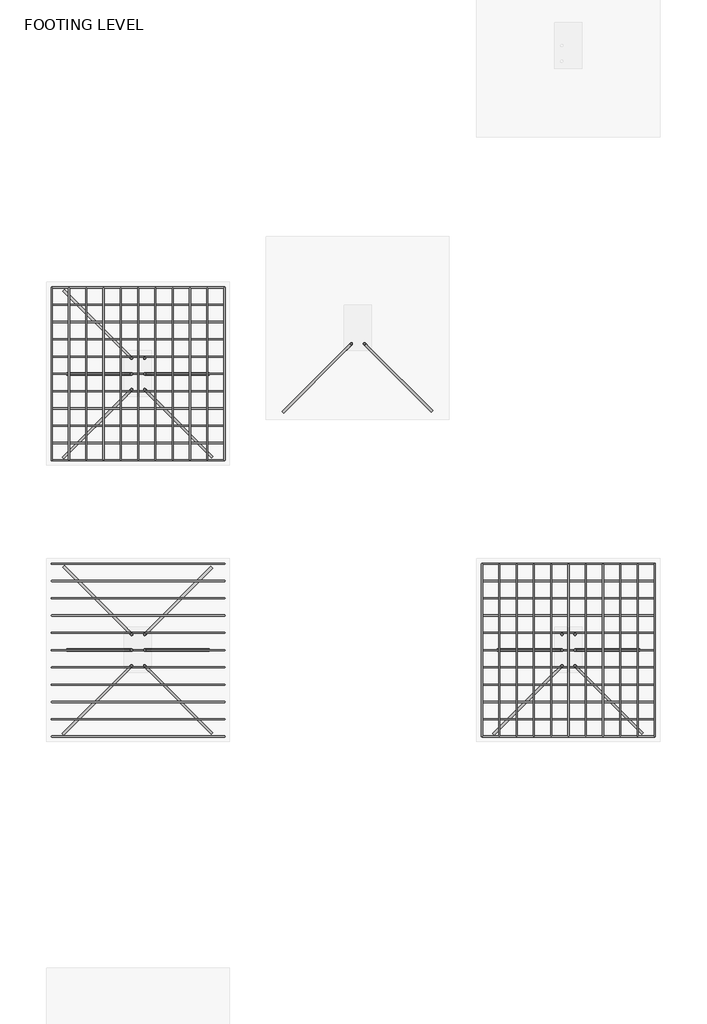
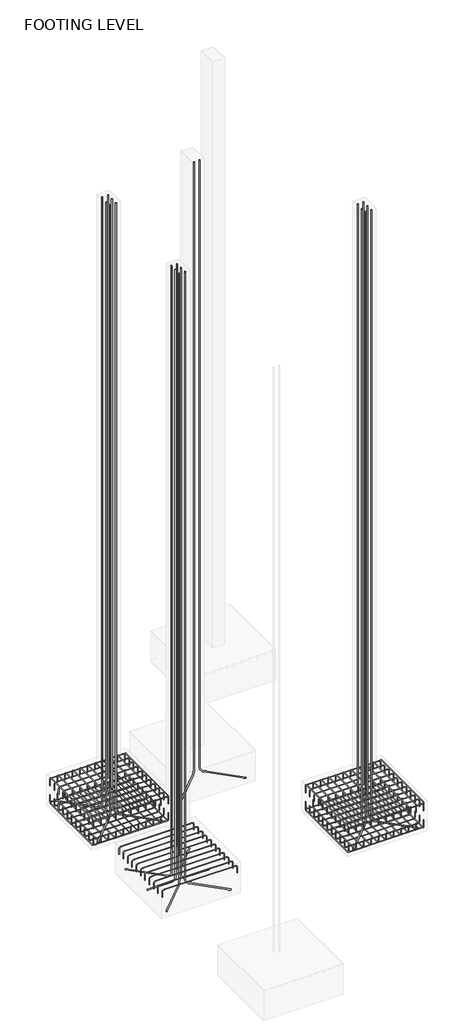
# One storey, part 6 of 10: 35 reinforcing bars.
"""IFC4 building model written with IfcOpenShell, lengths in millimetres."""

from ifc_helpers import new_model, si_unit, point, frame, origin, place, context, project, spatial, polyline, circle_curve, trimmed, segment, composite_curve, source, transform, mapped, element, save
from ifc_brep_helpers import swept_disk

model = new_model("IFC4")

# Units and contexts
model_context = context("Model", 3, world=origin())
ifc_project = project(units=[si_unit("LENGTHUNIT", "METRE", prefix="MILLI")], contexts=[model_context])

# Site, building, storey
site = spatial("IfcSite", under=ifc_project)
building = spatial("IfcBuilding", under=site)
storey = spatial("IfcBuildingStorey", under=building, Name="FOOTING LEVEL", Elevation=-1371.6)

# Reinforcing bars
placement = place(None, origin())
reinforcing_bar_shape = source(origin(), model_context, "Body", "SolidModel", [
    swept_disk(composite_curve([segment(polyline([(-3449.2793223, 2952.1203802, -1562.1), (-3449.2793223, 2952.1203802, -1447.8)]), True, "CONTINUOUS"), segment(trimmed(circle_curve(frame((-3449.2793223, 2985.4578802, -1447.8), z_axis=(-1.0, 0.0, 0.0), x_axis=(0.0, -33.33750000000009, 0.0)), 33.3375), [point((-3449.2793223, 2952.1203802, -1447.8))], [point((-3449.2793223, 2985.4578802, -1414.4625))], True, "CARTESIAN"), True, "CONTINUOUS"), segment(polyline([(-3449.2793223, 2985.4578802, -1414.4625), (-3449.2793223, 4357.0578802, -1414.4625)]), True, "CONTINUOUS"), segment(trimmed(circle_curve(frame((-3449.2793223, 4357.0578802, -1447.8), z_axis=(-1.0, 0.0, 0.0), x_axis=(0.0, 0.0, 33.337499999999864)), 33.3375), [point((-3449.2793223, 4357.0578802, -1414.4625))], [point((-3449.2793223, 4390.3953802, -1447.8))], True, "CARTESIAN"), True, "CONTINUOUS"), segment(polyline([(-3449.2793223, 4390.3953802, -1447.8), (-3449.2793223, 4390.3953802, -1562.1)]), True, "CONTINUOUS")], self_intersect=False), 4.7625),
])
element("IfcReinforcingBar", 1, at=placement, inside=storey, context=model_context, shape_type="MappedRepresentation", body=[
    mapped(reinforcing_bar_shape, transform((0.0, 0.0, 0.0), x_axis=(1.0, 0.0, 0.0), y_axis=(0.0, 1.0, 0.0), z_axis=(0.0, 0.0, 1.0))),
    mapped(reinforcing_bar_shape, transform((143.8275, 0.0, 0.0), x_axis=(1.0, 0.0, 0.0), y_axis=(0.0, 1.0, 0.0), z_axis=(0.0, 0.0, 1.0))),
    mapped(reinforcing_bar_shape, transform((287.655, 0.0, 0.0), x_axis=(1.0, 0.0, 0.0), y_axis=(0.0, 1.0, 0.0), z_axis=(0.0, 0.0, 1.0))),
    mapped(reinforcing_bar_shape, transform((431.4825, 0.0, 0.0), x_axis=(1.0, 0.0, 0.0), y_axis=(0.0, 1.0, 0.0), z_axis=(0.0, 0.0, 1.0))),
    mapped(reinforcing_bar_shape, transform((575.31, 0.0, 0.0), x_axis=(1.0, 0.0, 0.0), y_axis=(0.0, 1.0, 0.0), z_axis=(0.0, 0.0, 1.0))),
    mapped(reinforcing_bar_shape, transform((719.1375, 0.0, 0.0), x_axis=(1.0, 0.0, 0.0), y_axis=(0.0, 1.0, 0.0), z_axis=(0.0, 0.0, 1.0))),
    mapped(reinforcing_bar_shape, transform((862.965, 0.0, 0.0), x_axis=(1.0, 0.0, 0.0), y_axis=(0.0, 1.0, 0.0), z_axis=(0.0, 0.0, 1.0))),
    mapped(reinforcing_bar_shape, transform((1006.7925, 0.0, 0.0), x_axis=(1.0, 0.0, 0.0), y_axis=(0.0, 1.0, 0.0), z_axis=(0.0, 0.0, 1.0))),
    mapped(reinforcing_bar_shape, transform((1150.62, 0.0, 0.0), x_axis=(1.0, 0.0, 0.0), y_axis=(0.0, 1.0, 0.0), z_axis=(0.0, 0.0, 1.0))),
    mapped(reinforcing_bar_shape, transform((1294.4475, 0.0, 0.0), x_axis=(1.0, 0.0, 0.0), y_axis=(0.0, 1.0, 0.0), z_axis=(0.0, 0.0, 1.0))),
    mapped(reinforcing_bar_shape, transform((1438.275, 0.0, 0.0), x_axis=(1.0, 0.0, 0.0), y_axis=(0.0, 1.0, 0.0), z_axis=(0.0, 0.0, 1.0))),
])
reinforcing_bar_2_shape = source(origin(), model_context, "Body", "SolidModel", [
    swept_disk(composite_curve([segment(polyline([(-3449.2793223, 4390.3953802, -1790.7), (-3449.2793223, 4390.3953802, -1905.0)]), True, "CONTINUOUS"), segment(trimmed(circle_curve(frame((-3449.2793223, 4357.0578802, -1905.0), z_axis=(-1.0, 0.0, 0.0), x_axis=(0.0, 33.337499999999636, 0.0)), 33.3375), [point((-3449.2793223, 4390.3953802, -1905.0))], [point((-3449.2793223, 4357.0578802, -1938.3375))], True, "CARTESIAN"), True, "CONTINUOUS"), segment(polyline([(-3449.2793223, 4357.0578802, -1938.3375), (-3449.2793223, 2985.4578802, -1938.3375)]), True, "CONTINUOUS"), segment(trimmed(circle_curve(frame((-3449.2793223, 2985.4578802, -1905.0), z_axis=(-1.0, 0.0, 0.0), x_axis=(0.0, 0.0, -33.33750000000009)), 33.3375), [point((-3449.2793223, 2985.4578802, -1938.3375))], [point((-3449.2793223, 2952.1203802, -1905.0))], True, "CARTESIAN"), True, "CONTINUOUS"), segment(polyline([(-3449.2793223, 2952.1203802, -1905.0), (-3449.2793223, 2952.1203802, -1790.7)]), True, "CONTINUOUS")], self_intersect=False), 4.7625),
])
element("IfcReinforcingBar", 2, at=placement, inside=storey, context=model_context, shape_type="MappedRepresentation", body=[
    mapped(reinforcing_bar_2_shape, transform((0.0, 0.0, 0.0), x_axis=(1.0, 0.0, 0.0), y_axis=(0.0, 1.0, 0.0), z_axis=(0.0, 0.0, 1.0))),
    mapped(reinforcing_bar_2_shape, transform((143.8275, 0.0, 0.0), x_axis=(1.0, 0.0, 0.0), y_axis=(0.0, 1.0, 0.0), z_axis=(0.0, 0.0, 1.0))),
    mapped(reinforcing_bar_2_shape, transform((287.655, 0.0, 0.0), x_axis=(1.0, 0.0, 0.0), y_axis=(0.0, 1.0, 0.0), z_axis=(0.0, 0.0, 1.0))),
    mapped(reinforcing_bar_2_shape, transform((431.4825, 0.0, 0.0), x_axis=(1.0, 0.0, 0.0), y_axis=(0.0, 1.0, 0.0), z_axis=(0.0, 0.0, 1.0))),
    mapped(reinforcing_bar_2_shape, transform((575.31, 0.0, 0.0), x_axis=(1.0, 0.0, 0.0), y_axis=(0.0, 1.0, 0.0), z_axis=(0.0, 0.0, 1.0))),
    mapped(reinforcing_bar_2_shape, transform((719.1375, 0.0, 0.0), x_axis=(1.0, 0.0, 0.0), y_axis=(0.0, 1.0, 0.0), z_axis=(0.0, 0.0, 1.0))),
    mapped(reinforcing_bar_2_shape, transform((862.965, 0.0, 0.0), x_axis=(1.0, 0.0, 0.0), y_axis=(0.0, 1.0, 0.0), z_axis=(0.0, 0.0, 1.0))),
    mapped(reinforcing_bar_2_shape, transform((1006.7925, 0.0, 0.0), x_axis=(1.0, 0.0, 0.0), y_axis=(0.0, 1.0, 0.0), z_axis=(0.0, 0.0, 1.0))),
    mapped(reinforcing_bar_2_shape, transform((1150.62, 0.0, 0.0), x_axis=(1.0, 0.0, 0.0), y_axis=(0.0, 1.0, 0.0), z_axis=(0.0, 0.0, 1.0))),
    mapped(reinforcing_bar_2_shape, transform((1294.4475, 0.0, 0.0), x_axis=(1.0, 0.0, 0.0), y_axis=(0.0, 1.0, 0.0), z_axis=(0.0, 0.0, 1.0))),
    mapped(reinforcing_bar_2_shape, transform((1438.275, 0.0, 0.0), x_axis=(1.0, 0.0, 0.0), y_axis=(0.0, 1.0, 0.0), z_axis=(0.0, 0.0, 1.0))),
])
reinforcing_bar_3_shape = source(origin(), model_context, "Body", "SolidModel", [
    swept_disk(composite_curve([segment(polyline([(-2011.0043223, 4390.3953802, -1770.864029), (-2011.0043223, 4390.3953802, -1885.164029)]), True, "CONTINUOUS"), segment(trimmed(circle_curve(frame((-2044.3418223, 4390.3953802, -1885.164029), z_axis=(0.0, 1.0, 0.0), x_axis=(33.33750000000009, 0.0, 0.0)), 33.3375), [point((-2011.0043223, 4390.3953802, -1885.164029))], [point((-2044.3418223, 4390.3953802, -1918.501529))], True, "CARTESIAN"), True, "CONTINUOUS"), segment(polyline([(-2044.3418223, 4390.3953802, -1918.501529), (-3415.9418223, 4390.3953802, -1918.501529)]), True, "CONTINUOUS"), segment(trimmed(circle_curve(frame((-3415.9418223, 4390.3953802, -1885.164029), z_axis=(0.0, 1.0, 0.0), x_axis=(0.0, 0.0, -33.337499999999864)), 33.3375), [point((-3415.9418223, 4390.3953802, -1918.501529))], [point((-3449.2793223, 4390.3953802, -1885.164029))], True, "CARTESIAN"), True, "CONTINUOUS"), segment(polyline([(-3449.2793223, 4390.3953802, -1885.164029), (-3449.2793223, 4390.3953802, -1770.864029)]), True, "CONTINUOUS")], self_intersect=False), 4.7625),
])
element("IfcReinforcingBar", 3, at=placement, inside=storey, context=model_context, shape_type="MappedRepresentation", body=[
    mapped(reinforcing_bar_3_shape, transform((0.0, 0.0, 0.0), x_axis=(1.0, 0.0, 0.0), y_axis=(0.0, 1.0, 0.0), z_axis=(0.0, 0.0, 1.0))),
    mapped(reinforcing_bar_3_shape, transform((0.0, -143.8275, 0.0), x_axis=(1.0, 0.0, 0.0), y_axis=(0.0, 1.0, 0.0), z_axis=(0.0, 0.0, 1.0))),
    mapped(reinforcing_bar_3_shape, transform((0.0, -287.655, 0.0), x_axis=(1.0, 0.0, 0.0), y_axis=(0.0, 1.0, 0.0), z_axis=(0.0, 0.0, 1.0))),
    mapped(reinforcing_bar_3_shape, transform((0.0, -431.4825, 0.0), x_axis=(1.0, 0.0, 0.0), y_axis=(0.0, 1.0, 0.0), z_axis=(0.0, 0.0, 1.0))),
    mapped(reinforcing_bar_3_shape, transform((0.0, -575.31, 0.0), x_axis=(1.0, 0.0, 0.0), y_axis=(0.0, 1.0, 0.0), z_axis=(0.0, 0.0, 1.0))),
    mapped(reinforcing_bar_3_shape, transform((0.0, -719.1375, 0.0), x_axis=(1.0, 0.0, 0.0), y_axis=(0.0, 1.0, 0.0), z_axis=(0.0, 0.0, 1.0))),
    mapped(reinforcing_bar_3_shape, transform((0.0, -862.965, 0.0), x_axis=(1.0, 0.0, 0.0), y_axis=(0.0, 1.0, 0.0), z_axis=(0.0, 0.0, 1.0))),
    mapped(reinforcing_bar_3_shape, transform((0.0, -1006.7925, 0.0), x_axis=(1.0, 0.0, 0.0), y_axis=(0.0, 1.0, 0.0), z_axis=(0.0, 0.0, 1.0))),
    mapped(reinforcing_bar_3_shape, transform((0.0, -1150.62, 0.0), x_axis=(1.0, 0.0, 0.0), y_axis=(0.0, 1.0, 0.0), z_axis=(0.0, 0.0, 1.0))),
    mapped(reinforcing_bar_3_shape, transform((0.0, -1294.4475, 0.0), x_axis=(1.0, 0.0, 0.0), y_axis=(0.0, 1.0, 0.0), z_axis=(0.0, 0.0, 1.0))),
    mapped(reinforcing_bar_3_shape, transform((0.0, -1438.275, 0.0), x_axis=(1.0, 0.0, 0.0), y_axis=(0.0, 1.0, 0.0), z_axis=(0.0, 0.0, 1.0))),
])
reinforcing_bar_4_shape = source(origin(), model_context, "Body", "SolidModel", [
    swept_disk(composite_curve([segment(polyline([(-2011.0043223, 2952.1203802, -1586.5406765), (-2011.0043223, 2952.1203802, -1472.2406765)]), True, "CONTINUOUS"), segment(trimmed(circle_curve(frame((-2044.3418223, 2952.1203802, -1472.2406765), z_axis=(0.0, -1.0, 0.0), x_axis=(33.33750000000009, 0.0, 0.0)), 33.3375), [point((-2011.0043223, 2952.1203802, -1472.2406765))], [point((-2044.3418223, 2952.1203802, -1438.9031765))], True, "CARTESIAN"), True, "CONTINUOUS"), segment(polyline([(-2044.3418223, 2952.1203802, -1438.9031765), (-3415.9418223, 2952.1203802, -1438.9031765)]), True, "CONTINUOUS"), segment(trimmed(circle_curve(frame((-3415.9418223, 2952.1203802, -1472.2406765), z_axis=(0.0, -1.0, 0.0), x_axis=(0.0, 0.0, 33.33750000000009)), 33.3375), [point((-3415.9418223, 2952.1203802, -1438.9031765))], [point((-3449.2793223, 2952.1203802, -1472.2406765))], True, "CARTESIAN"), True, "CONTINUOUS"), segment(polyline([(-3449.2793223, 2952.1203802, -1472.2406765), (-3449.2793223, 2952.1203802, -1586.5406765)]), True, "CONTINUOUS")], self_intersect=False), 4.7625),
])
element("IfcReinforcingBar", 4, at=placement, inside=storey, context=model_context, shape_type="MappedRepresentation", body=[
    mapped(reinforcing_bar_4_shape, transform((0.0, 0.0, 0.0), x_axis=(1.0, 0.0, 0.0), y_axis=(0.0, 1.0, 0.0), z_axis=(0.0, 0.0, 1.0))),
    mapped(reinforcing_bar_4_shape, transform((0.0, 143.8275, 0.0), x_axis=(1.0, 0.0, 0.0), y_axis=(0.0, 1.0, 0.0), z_axis=(0.0, 0.0, 1.0))),
    mapped(reinforcing_bar_4_shape, transform((0.0, 287.655, 0.0), x_axis=(1.0, 0.0, 0.0), y_axis=(0.0, 1.0, 0.0), z_axis=(0.0, 0.0, 1.0))),
    mapped(reinforcing_bar_4_shape, transform((0.0, 431.4825, 0.0), x_axis=(1.0, 0.0, 0.0), y_axis=(0.0, 1.0, 0.0), z_axis=(0.0, 0.0, 1.0))),
    mapped(reinforcing_bar_4_shape, transform((0.0, 575.31, 0.0), x_axis=(1.0, 0.0, 0.0), y_axis=(0.0, 1.0, 0.0), z_axis=(0.0, 0.0, 1.0))),
    mapped(reinforcing_bar_4_shape, transform((0.0, 719.1375, 0.0), x_axis=(1.0, 0.0, 0.0), y_axis=(0.0, 1.0, 0.0), z_axis=(0.0, 0.0, 1.0))),
    mapped(reinforcing_bar_4_shape, transform((0.0, 862.965, 0.0), x_axis=(1.0, 0.0, 0.0), y_axis=(0.0, 1.0, 0.0), z_axis=(0.0, 0.0, 1.0))),
    mapped(reinforcing_bar_4_shape, transform((0.0, 1006.7925, 0.0), x_axis=(1.0, 0.0, 0.0), y_axis=(0.0, 1.0, 0.0), z_axis=(0.0, 0.0, 1.0))),
    mapped(reinforcing_bar_4_shape, transform((0.0, 1150.62, 0.0), x_axis=(1.0, 0.0, 0.0), y_axis=(0.0, 1.0, 0.0), z_axis=(0.0, 0.0, 1.0))),
    mapped(reinforcing_bar_4_shape, transform((0.0, 1294.4475, 0.0), x_axis=(1.0, 0.0, 0.0), y_axis=(0.0, 1.0, 0.0), z_axis=(0.0, 0.0, 1.0))),
    mapped(reinforcing_bar_4_shape, transform((0.0, 1438.275, 0.0), x_axis=(1.0, 0.0, 0.0), y_axis=(0.0, 1.0, 0.0), z_axis=(0.0, 0.0, 1.0))),
])
reinforcing_bar_5_shape = source(origin(), model_context, "Body", "SolidModel", [
    swept_disk(composite_curve([segment(polyline([(-7030.6793223, 5250.8203802, -1562.1), (-7030.6793223, 5250.8203802, -1447.8)]), True, "CONTINUOUS"), segment(trimmed(circle_curve(frame((-7030.6793223, 5284.1578802, -1447.8), z_axis=(-1.0, 0.0, 0.0), x_axis=(0.0, -33.337500000000546, 0.0)), 33.3375), [point((-7030.6793223, 5250.8203802, -1447.8))], [point((-7030.6793223, 5284.1578802, -1414.4625))], True, "CARTESIAN"), True, "CONTINUOUS"), segment(polyline([(-7030.6793223, 5284.1578802, -1414.4625), (-7030.6793223, 6655.7578802, -1414.4625)]), True, "CONTINUOUS"), segment(trimmed(circle_curve(frame((-7030.6793223, 6655.7578802, -1447.8), z_axis=(-1.0, 0.0, 0.0), x_axis=(0.0, 0.0, 33.337499999999864)), 33.3375), [point((-7030.6793223, 6655.7578802, -1414.4625))], [point((-7030.6793223, 6689.0953802, -1447.8))], True, "CARTESIAN"), True, "CONTINUOUS"), segment(polyline([(-7030.6793223, 6689.0953802, -1447.8), (-7030.6793223, 6689.0953802, -1562.1)]), True, "CONTINUOUS")], self_intersect=False), 4.7625),
])
element("IfcReinforcingBar", 5, at=placement, inside=storey, context=model_context, shape_type="MappedRepresentation", body=[
    mapped(reinforcing_bar_5_shape, transform((0.0, 0.0, 0.0), x_axis=(1.0, 0.0, 0.0), y_axis=(0.0, 1.0, 0.0), z_axis=(0.0, 0.0, 1.0))),
    mapped(reinforcing_bar_5_shape, transform((143.8275, 0.0, 0.0), x_axis=(1.0, 0.0, 0.0), y_axis=(0.0, 1.0, 0.0), z_axis=(0.0, 0.0, 1.0))),
    mapped(reinforcing_bar_5_shape, transform((287.655, 0.0, 0.0), x_axis=(1.0, 0.0, 0.0), y_axis=(0.0, 1.0, 0.0), z_axis=(0.0, 0.0, 1.0))),
    mapped(reinforcing_bar_5_shape, transform((431.4825, 0.0, 0.0), x_axis=(1.0, 0.0, 0.0), y_axis=(0.0, 1.0, 0.0), z_axis=(0.0, 0.0, 1.0))),
    mapped(reinforcing_bar_5_shape, transform((575.31, 0.0, 0.0), x_axis=(1.0, 0.0, 0.0), y_axis=(0.0, 1.0, 0.0), z_axis=(0.0, 0.0, 1.0))),
    mapped(reinforcing_bar_5_shape, transform((719.1375, 0.0, 0.0), x_axis=(1.0, 0.0, 0.0), y_axis=(0.0, 1.0, 0.0), z_axis=(0.0, 0.0, 1.0))),
    mapped(reinforcing_bar_5_shape, transform((862.965, 0.0, 0.0), x_axis=(1.0, 0.0, 0.0), y_axis=(0.0, 1.0, 0.0), z_axis=(0.0, 0.0, 1.0))),
    mapped(reinforcing_bar_5_shape, transform((1006.7925, 0.0, 0.0), x_axis=(1.0, 0.0, 0.0), y_axis=(0.0, 1.0, 0.0), z_axis=(0.0, 0.0, 1.0))),
    mapped(reinforcing_bar_5_shape, transform((1150.62, 0.0, 0.0), x_axis=(1.0, 0.0, 0.0), y_axis=(0.0, 1.0, 0.0), z_axis=(0.0, 0.0, 1.0))),
    mapped(reinforcing_bar_5_shape, transform((1294.4475, 0.0, 0.0), x_axis=(1.0, 0.0, 0.0), y_axis=(0.0, 1.0, 0.0), z_axis=(0.0, 0.0, 1.0))),
    mapped(reinforcing_bar_5_shape, transform((1438.275, 0.0, 0.0), x_axis=(1.0, 0.0, 0.0), y_axis=(0.0, 1.0, 0.0), z_axis=(0.0, 0.0, 1.0))),
])
reinforcing_bar_6_shape = source(origin(), model_context, "Body", "SolidModel", [
    swept_disk(composite_curve([segment(polyline([(-7030.6793223, 6689.0953802, -1790.7), (-7030.6793223, 6689.0953802, -1905.0)]), True, "CONTINUOUS"), segment(trimmed(circle_curve(frame((-7030.6793223, 6655.7578802, -1905.0), z_axis=(-1.0, 0.0, 0.0), x_axis=(0.0, 33.337500000000546, 0.0)), 33.3375), [point((-7030.6793223, 6689.0953802, -1905.0))], [point((-7030.6793223, 6655.7578802, -1938.3375))], True, "CARTESIAN"), True, "CONTINUOUS"), segment(polyline([(-7030.6793223, 6655.7578802, -1938.3375), (-7030.6793223, 5284.1578802, -1938.3375)]), True, "CONTINUOUS"), segment(trimmed(circle_curve(frame((-7030.6793223, 5284.1578802, -1905.0), z_axis=(-1.0, 0.0, 0.0), x_axis=(0.0, 0.0, -33.33750000000009)), 33.3375), [point((-7030.6793223, 5284.1578802, -1938.3375))], [point((-7030.6793223, 5250.8203802, -1905.0))], True, "CARTESIAN"), True, "CONTINUOUS"), segment(polyline([(-7030.6793223, 5250.8203802, -1905.0), (-7030.6793223, 5250.8203802, -1790.7)]), True, "CONTINUOUS")], self_intersect=False), 4.7625),
])
element("IfcReinforcingBar", 6, at=placement, inside=storey, context=model_context, shape_type="MappedRepresentation", body=[
    mapped(reinforcing_bar_6_shape, transform((0.0, 0.0, 0.0), x_axis=(1.0, 0.0, 0.0), y_axis=(0.0, 1.0, 0.0), z_axis=(0.0, 0.0, 1.0))),
    mapped(reinforcing_bar_6_shape, transform((143.8275, 0.0, 0.0), x_axis=(1.0, 0.0, 0.0), y_axis=(0.0, 1.0, 0.0), z_axis=(0.0, 0.0, 1.0))),
    mapped(reinforcing_bar_6_shape, transform((287.655, 0.0, 0.0), x_axis=(1.0, 0.0, 0.0), y_axis=(0.0, 1.0, 0.0), z_axis=(0.0, 0.0, 1.0))),
    mapped(reinforcing_bar_6_shape, transform((431.4825, 0.0, 0.0), x_axis=(1.0, 0.0, 0.0), y_axis=(0.0, 1.0, 0.0), z_axis=(0.0, 0.0, 1.0))),
    mapped(reinforcing_bar_6_shape, transform((575.31, 0.0, 0.0), x_axis=(1.0, 0.0, 0.0), y_axis=(0.0, 1.0, 0.0), z_axis=(0.0, 0.0, 1.0))),
    mapped(reinforcing_bar_6_shape, transform((719.1375, 0.0, 0.0), x_axis=(1.0, 0.0, 0.0), y_axis=(0.0, 1.0, 0.0), z_axis=(0.0, 0.0, 1.0))),
    mapped(reinforcing_bar_6_shape, transform((862.965, 0.0, 0.0), x_axis=(1.0, 0.0, 0.0), y_axis=(0.0, 1.0, 0.0), z_axis=(0.0, 0.0, 1.0))),
    mapped(reinforcing_bar_6_shape, transform((1006.7925, 0.0, 0.0), x_axis=(1.0, 0.0, 0.0), y_axis=(0.0, 1.0, 0.0), z_axis=(0.0, 0.0, 1.0))),
    mapped(reinforcing_bar_6_shape, transform((1150.62, 0.0, 0.0), x_axis=(1.0, 0.0, 0.0), y_axis=(0.0, 1.0, 0.0), z_axis=(0.0, 0.0, 1.0))),
    mapped(reinforcing_bar_6_shape, transform((1294.4475, 0.0, 0.0), x_axis=(1.0, 0.0, 0.0), y_axis=(0.0, 1.0, 0.0), z_axis=(0.0, 0.0, 1.0))),
    mapped(reinforcing_bar_6_shape, transform((1438.275, 0.0, 0.0), x_axis=(1.0, 0.0, 0.0), y_axis=(0.0, 1.0, 0.0), z_axis=(0.0, 0.0, 1.0))),
])
reinforcing_bar_7_shape = source(origin(), model_context, "Body", "SolidModel", [
    swept_disk(composite_curve([segment(polyline([(-5592.4043223, 6689.0953802, -1770.864029), (-5592.4043223, 6689.0953802, -1885.164029)]), True, "CONTINUOUS"), segment(trimmed(circle_curve(frame((-5625.7418223, 6689.0953802, -1885.164029), z_axis=(0.0, 1.0, 0.0), x_axis=(33.337500000000546, 0.0, 0.0)), 33.3375), [point((-5592.4043223, 6689.0953802, -1885.164029))], [point((-5625.7418223, 6689.0953802, -1918.501529))], True, "CARTESIAN"), True, "CONTINUOUS"), segment(polyline([(-5625.7418223, 6689.0953802, -1918.501529), (-6997.3418223, 6689.0953802, -1918.501529)]), True, "CONTINUOUS"), segment(trimmed(circle_curve(frame((-6997.3418223, 6689.0953802, -1885.164029), z_axis=(0.0, 1.0, 0.0), x_axis=(0.0, 0.0, -33.337499999999864)), 33.3375), [point((-6997.3418223, 6689.0953802, -1918.501529))], [point((-7030.6793223, 6689.0953802, -1885.164029))], True, "CARTESIAN"), True, "CONTINUOUS"), segment(polyline([(-7030.6793223, 6689.0953802, -1885.164029), (-7030.6793223, 6689.0953802, -1770.864029)]), True, "CONTINUOUS")], self_intersect=False), 4.7625),
])
element("IfcReinforcingBar", 7, at=placement, inside=storey, context=model_context, shape_type="MappedRepresentation", body=[
    mapped(reinforcing_bar_7_shape, transform((0.0, 0.0, 0.0), x_axis=(1.0, 0.0, 0.0), y_axis=(0.0, 1.0, 0.0), z_axis=(0.0, 0.0, 1.0))),
    mapped(reinforcing_bar_7_shape, transform((0.0, -143.8275, 0.0), x_axis=(1.0, 0.0, 0.0), y_axis=(0.0, 1.0, 0.0), z_axis=(0.0, 0.0, 1.0))),
    mapped(reinforcing_bar_7_shape, transform((0.0, -287.655, 0.0), x_axis=(1.0, 0.0, 0.0), y_axis=(0.0, 1.0, 0.0), z_axis=(0.0, 0.0, 1.0))),
    mapped(reinforcing_bar_7_shape, transform((0.0, -431.4825, 0.0), x_axis=(1.0, 0.0, 0.0), y_axis=(0.0, 1.0, 0.0), z_axis=(0.0, 0.0, 1.0))),
    mapped(reinforcing_bar_7_shape, transform((0.0, -575.31, 0.0), x_axis=(1.0, 0.0, 0.0), y_axis=(0.0, 1.0, 0.0), z_axis=(0.0, 0.0, 1.0))),
    mapped(reinforcing_bar_7_shape, transform((0.0, -719.1375, 0.0), x_axis=(1.0, 0.0, 0.0), y_axis=(0.0, 1.0, 0.0), z_axis=(0.0, 0.0, 1.0))),
    mapped(reinforcing_bar_7_shape, transform((0.0, -862.965, 0.0), x_axis=(1.0, 0.0, 0.0), y_axis=(0.0, 1.0, 0.0), z_axis=(0.0, 0.0, 1.0))),
    mapped(reinforcing_bar_7_shape, transform((0.0, -1006.7925, 0.0), x_axis=(1.0, 0.0, 0.0), y_axis=(0.0, 1.0, 0.0), z_axis=(0.0, 0.0, 1.0))),
    mapped(reinforcing_bar_7_shape, transform((0.0, -1150.62, 0.0), x_axis=(1.0, 0.0, 0.0), y_axis=(0.0, 1.0, 0.0), z_axis=(0.0, 0.0, 1.0))),
    mapped(reinforcing_bar_7_shape, transform((0.0, -1294.4475, 0.0), x_axis=(1.0, 0.0, 0.0), y_axis=(0.0, 1.0, 0.0), z_axis=(0.0, 0.0, 1.0))),
    mapped(reinforcing_bar_7_shape, transform((0.0, -1438.275, 0.0), x_axis=(1.0, 0.0, 0.0), y_axis=(0.0, 1.0, 0.0), z_axis=(0.0, 0.0, 1.0))),
])
reinforcing_bar_8_shape = source(origin(), model_context, "Body", "SolidModel", [
    swept_disk(composite_curve([segment(polyline([(-5592.4043223, 5250.8203802, -1586.5406765), (-5592.4043223, 5250.8203802, -1472.2406765)]), True, "CONTINUOUS"), segment(trimmed(circle_curve(frame((-5625.7418223, 5250.8203802, -1472.2406765), z_axis=(0.0, -1.0, 0.0), x_axis=(33.337500000000546, 0.0, 0.0)), 33.3375), [point((-5592.4043223, 5250.8203802, -1472.2406765))], [point((-5625.7418223, 5250.8203802, -1438.9031765))], True, "CARTESIAN"), True, "CONTINUOUS"), segment(polyline([(-5625.7418223, 5250.8203802, -1438.9031765), (-6997.3418223, 5250.8203802, -1438.9031765)]), True, "CONTINUOUS"), segment(trimmed(circle_curve(frame((-6997.3418223, 5250.8203802, -1472.2406765), z_axis=(0.0, -1.0, 0.0), x_axis=(0.0, 0.0, 33.33750000000009)), 33.3375), [point((-6997.3418223, 5250.8203802, -1438.9031765))], [point((-7030.6793223, 5250.8203802, -1472.2406765))], True, "CARTESIAN"), True, "CONTINUOUS"), segment(polyline([(-7030.6793223, 5250.8203802, -1472.2406765), (-7030.6793223, 5250.8203802, -1586.5406765)]), True, "CONTINUOUS")], self_intersect=False), 4.7625),
])
element("IfcReinforcingBar", 8, at=placement, inside=storey, context=model_context, shape_type="MappedRepresentation", body=[
    mapped(reinforcing_bar_8_shape, transform((0.0, 0.0, 0.0), x_axis=(1.0, 0.0, 0.0), y_axis=(0.0, 1.0, 0.0), z_axis=(0.0, 0.0, 1.0))),
    mapped(reinforcing_bar_8_shape, transform((0.0, 143.8275, 0.0), x_axis=(1.0, 0.0, 0.0), y_axis=(0.0, 1.0, 0.0), z_axis=(0.0, 0.0, 1.0))),
    mapped(reinforcing_bar_8_shape, transform((0.0, 287.655, 0.0), x_axis=(1.0, 0.0, 0.0), y_axis=(0.0, 1.0, 0.0), z_axis=(0.0, 0.0, 1.0))),
    mapped(reinforcing_bar_8_shape, transform((0.0, 431.4825, 0.0), x_axis=(1.0, 0.0, 0.0), y_axis=(0.0, 1.0, 0.0), z_axis=(0.0, 0.0, 1.0))),
    mapped(reinforcing_bar_8_shape, transform((0.0, 575.31, 0.0), x_axis=(1.0, 0.0, 0.0), y_axis=(0.0, 1.0, 0.0), z_axis=(0.0, 0.0, 1.0))),
    mapped(reinforcing_bar_8_shape, transform((0.0, 719.1375, 0.0), x_axis=(1.0, 0.0, 0.0), y_axis=(0.0, 1.0, 0.0), z_axis=(0.0, 0.0, 1.0))),
    mapped(reinforcing_bar_8_shape, transform((0.0, 862.965, 0.0), x_axis=(1.0, 0.0, 0.0), y_axis=(0.0, 1.0, 0.0), z_axis=(0.0, 0.0, 1.0))),
    mapped(reinforcing_bar_8_shape, transform((0.0, 1006.7925, 0.0), x_axis=(1.0, 0.0, 0.0), y_axis=(0.0, 1.0, 0.0), z_axis=(0.0, 0.0, 1.0))),
    mapped(reinforcing_bar_8_shape, transform((0.0, 1150.62, 0.0), x_axis=(1.0, 0.0, 0.0), y_axis=(0.0, 1.0, 0.0), z_axis=(0.0, 0.0, 1.0))),
    mapped(reinforcing_bar_8_shape, transform((0.0, 1294.4475, 0.0), x_axis=(1.0, 0.0, 0.0), y_axis=(0.0, 1.0, 0.0), z_axis=(0.0, 0.0, 1.0))),
    mapped(reinforcing_bar_8_shape, transform((0.0, 1438.275, 0.0), x_axis=(1.0, 0.0, 0.0), y_axis=(0.0, 1.0, 0.0), z_axis=(0.0, 0.0, 1.0))),
])
reinforcing_bar_9_shape = source(origin(), model_context, "Body", "SolidModel", [
    swept_disk(composite_curve([segment(polyline([(-5592.4043223, 2952.1203802, -1586.5406765), (-5592.4043223, 2952.1203802, -1472.2406765)]), True, "CONTINUOUS"), segment(trimmed(circle_curve(frame((-5625.7418223, 2952.1203802, -1472.2406765), z_axis=(0.0, -1.0, 0.0), x_axis=(33.337500000000546, 0.0, 0.0)), 33.3375), [point((-5592.4043223, 2952.1203802, -1472.2406765))], [point((-5625.7418223, 2952.1203802, -1438.9031765))], True, "CARTESIAN"), True, "CONTINUOUS"), segment(polyline([(-5625.7418223, 2952.1203802, -1438.9031765), (-6997.3418223, 2952.1203802, -1438.9031765)]), True, "CONTINUOUS"), segment(trimmed(circle_curve(frame((-6997.3418223, 2952.1203802, -1472.2406765), z_axis=(0.0, -1.0, 0.0), x_axis=(0.0, 0.0, 33.33750000000009)), 33.3375), [point((-6997.3418223, 2952.1203802, -1438.9031765))], [point((-7030.6793223, 2952.1203802, -1472.2406765))], True, "CARTESIAN"), True, "CONTINUOUS"), segment(polyline([(-7030.6793223, 2952.1203802, -1472.2406765), (-7030.6793223, 2952.1203802, -1586.5406765)]), True, "CONTINUOUS")], self_intersect=False), 4.7625),
])
element("IfcReinforcingBar", 9, at=placement, inside=storey, context=model_context, shape_type="MappedRepresentation", body=[
    mapped(reinforcing_bar_9_shape, transform((0.0, 0.0, 0.0), x_axis=(1.0, 0.0, 0.0), y_axis=(0.0, 1.0, 0.0), z_axis=(0.0, 0.0, 1.0))),
    mapped(reinforcing_bar_9_shape, transform((0.0, 143.8275, 0.0), x_axis=(1.0, 0.0, 0.0), y_axis=(0.0, 1.0, 0.0), z_axis=(0.0, 0.0, 1.0))),
    mapped(reinforcing_bar_9_shape, transform((0.0, 287.655, 0.0), x_axis=(1.0, 0.0, 0.0), y_axis=(0.0, 1.0, 0.0), z_axis=(0.0, 0.0, 1.0))),
    mapped(reinforcing_bar_9_shape, transform((0.0, 431.4825, 0.0), x_axis=(1.0, 0.0, 0.0), y_axis=(0.0, 1.0, 0.0), z_axis=(0.0, 0.0, 1.0))),
    mapped(reinforcing_bar_9_shape, transform((0.0, 575.31, 0.0), x_axis=(1.0, 0.0, 0.0), y_axis=(0.0, 1.0, 0.0), z_axis=(0.0, 0.0, 1.0))),
    mapped(reinforcing_bar_9_shape, transform((0.0, 719.1375, 0.0), x_axis=(1.0, 0.0, 0.0), y_axis=(0.0, 1.0, 0.0), z_axis=(0.0, 0.0, 1.0))),
    mapped(reinforcing_bar_9_shape, transform((0.0, 862.965, 0.0), x_axis=(1.0, 0.0, 0.0), y_axis=(0.0, 1.0, 0.0), z_axis=(0.0, 0.0, 1.0))),
    mapped(reinforcing_bar_9_shape, transform((0.0, 1006.7925, 0.0), x_axis=(1.0, 0.0, 0.0), y_axis=(0.0, 1.0, 0.0), z_axis=(0.0, 0.0, 1.0))),
    mapped(reinforcing_bar_9_shape, transform((0.0, 1150.62, 0.0), x_axis=(1.0, 0.0, 0.0), y_axis=(0.0, 1.0, 0.0), z_axis=(0.0, 0.0, 1.0))),
    mapped(reinforcing_bar_9_shape, transform((0.0, 1294.4475, 0.0), x_axis=(1.0, 0.0, 0.0), y_axis=(0.0, 1.0, 0.0), z_axis=(0.0, 0.0, 1.0))),
    mapped(reinforcing_bar_9_shape, transform((0.0, 1438.275, 0.0), x_axis=(1.0, 0.0, 0.0), y_axis=(0.0, 1.0, 0.0), z_axis=(0.0, 0.0, 1.0))),
])
element("IfcReinforcingBar", 10, at=placement, inside=storey, context=model_context, shape_type="SolidModel", body=[
    swept_disk(composite_curve([segment(polyline([(-6365.9020144, 3540.6976881, -1333.5), (-6365.9020144, 3540.6976881, 10477.5)]), True, "CONTINUOUS")], self_intersect=False), 9.525),
])
element("IfcReinforcingBar", 11, at=placement, inside=storey, context=model_context, shape_type="SolidModel", body=[
    swept_disk(composite_curve([segment(polyline([(-6257.1816302, 3801.8180723, -1333.5), (-6257.1816302, 3801.8180723, 10477.5)]), True, "CONTINUOUS")], self_intersect=False), 9.525),
])
element("IfcReinforcingBar", 12, at=placement, inside=storey, context=model_context, shape_type="SolidModel", body=[
    swept_disk(composite_curve([segment(polyline([(-6365.9020144, 3801.8180723, -1333.5), (-6365.9020144, 3801.8180723, 10477.5)]), True, "CONTINUOUS")], self_intersect=False), 9.525),
])
element("IfcReinforcingBar", 13, at=placement, inside=storey, context=model_context, shape_type="SolidModel", body=[
    swept_disk(composite_curve([segment(polyline([(-5695.5058743, 2979.0219322, -1910.4342608), (-6210.0352856, 3493.5513434, -1910.4342608)]), True, "CONTINUOUS"), segment(trimmed(circle_curve(frame((-6210.0352856, 3493.5513434, -1843.7592608), z_axis=(0.7071067811865758, 0.7071067811865194, 0.0), x_axis=(0.0, 0.0, -66.67499999999995)), 66.675), [point((-6210.0352856, 3493.5513434, -1910.4342608))], [point((-6257.1816302, 3540.6976881, -1843.7592608))], True, "CARTESIAN"), True, "CONTINUOUS"), segment(polyline([(-6257.1816302, 3540.6976881, -1843.7592608), (-6257.1816302, 3540.6976881, 10477.5)]), True, "CONTINUOUS")], self_intersect=False), 9.525),
])
element("IfcReinforcingBar", 14, at=placement, inside=storey, context=model_context, shape_type="SolidModel", body=[
    swept_disk(composite_curve([segment(polyline([(-6935.5961481, 2971.0035544, -1910.4342608), (-6413.048359, 3493.5513434, -1910.4342608)]), True, "CONTINUOUS"), segment(trimmed(circle_curve(frame((-6413.048359, 3493.5513434, -1843.7592608), z_axis=(0.707106781186569, -0.707106781186526, 0.0), x_axis=(0.0, 0.0, -66.67499999999995)), 66.675), [point((-6413.048359, 3493.5513434, -1910.4342608))], [point((-6365.9020144, 3540.6976881, -1843.7592608))], True, "CARTESIAN"), True, "CONTINUOUS"), segment(polyline([(-6365.9020144, 3540.6976881, -1843.7592608), (-6365.9020144, 3540.6976881, 10477.5)]), True, "CONTINUOUS")], self_intersect=False), 9.525),
])
element("IfcReinforcingBar", 15, at=placement, inside=storey, context=model_context, shape_type="SolidModel", body=[
    swept_disk(composite_curve([segment(polyline([(-5698.4625098, 4360.5371927, -1910.4342608), (-6210.0352856, 3848.9644169, -1910.4342608)]), True, "CONTINUOUS"), segment(trimmed(circle_curve(frame((-6210.0352856, 3848.9644169, -1843.7592608), z_axis=(-0.7071067811865738, 0.7071067811865214, 0.0), x_axis=(0.0, 0.0, -66.67499999999995)), 66.675), [point((-6210.0352856, 3848.9644169, -1910.4342608))], [point((-6257.1816302, 3801.8180723, -1843.7592608))], True, "CARTESIAN"), True, "CONTINUOUS"), segment(polyline([(-6257.1816302, 3801.8180723, -1843.7592608), (-6257.1816302, 3801.8180723, 10477.5)]), True, "CONTINUOUS")], self_intersect=False), 9.525),
])
element("IfcReinforcingBar", 16, at=placement, inside=storey, context=model_context, shape_type="SolidModel", body=[
    swept_disk(composite_curve([segment(polyline([(-6930.0808347, 4365.9968926, -1910.4342608), (-6413.048359, 3848.9644169, -1910.4342608)]), True, "CONTINUOUS"), segment(trimmed(circle_curve(frame((-6413.048359, 3848.9644169, -1843.7592608), z_axis=(-0.7071067811865711, -0.7071067811865239, 0.0), x_axis=(0.0, 0.0, -66.67499999999995)), 66.675), [point((-6413.048359, 3848.9644169, -1910.4342608))], [point((-6365.9020144, 3801.8180723, -1843.7592608))], True, "CARTESIAN"), True, "CONTINUOUS"), segment(polyline([(-6365.9020144, 3801.8180723, -1843.7592608), (-6365.9020144, 3801.8180723, 10477.5)]), True, "CONTINUOUS")], self_intersect=False), 9.525),
])
element("IfcReinforcingBar", 17, at=placement, inside=storey, context=model_context, shape_type="SolidModel", body=[
    swept_disk(composite_curve([segment(polyline([(-5718.9517538, 3671.2578802, -1910.4342608), (-6190.5066302, 3671.2578802, -1910.4342608)]), True, "CONTINUOUS"), segment(trimmed(circle_curve(frame((-6190.5066302, 3671.2578802, -1843.7592608), z_axis=(0.0, 1.0, 0.0), x_axis=(0.0, 0.0, -66.67499999999995)), 66.675), [point((-6190.5066302, 3671.2578802, -1910.4342608))], [point((-6257.1816302, 3671.2578802, -1843.7592608))], True, "CARTESIAN"), True, "CONTINUOUS"), segment(polyline([(-6257.1816302, 3671.2578802, -1843.7592608), (-6257.1816302, 3671.2578802, 10477.5)]), True, "CONTINUOUS")], self_intersect=False), 9.525),
])
element("IfcReinforcingBar", 18, at=placement, inside=storey, context=model_context, shape_type="SolidModel", body=[
    swept_disk(composite_curve([segment(polyline([(-6904.1318909, 3671.2578802, -1910.4342608), (-6432.5770144, 3671.2578802, -1910.4342608)]), True, "CONTINUOUS"), segment(trimmed(circle_curve(frame((-6432.5770144, 3671.2578802, -1843.7592608), z_axis=(0.0, -1.0, 0.0), x_axis=(0.0, 0.0, -66.67499999999995)), 66.675), [point((-6432.5770144, 3671.2578802, -1910.4342608))], [point((-6365.9020144, 3671.2578802, -1843.7592608))], True, "CARTESIAN"), True, "CONTINUOUS"), segment(polyline([(-6365.9020144, 3671.2578802, -1843.7592608), (-6365.9020144, 3671.2578802, 10477.5)]), True, "CONTINUOUS")], self_intersect=False), 9.525),
])
element("IfcReinforcingBar", 19, at=placement, inside=storey, context=model_context, shape_type="SolidModel", body=[
    swept_disk(composite_curve([segment(polyline([(-2784.5020144, 3540.6976881, -1333.5), (-2784.5020144, 3540.6976881, 10477.5)]), True, "CONTINUOUS")], self_intersect=False), 9.525),
])
element("IfcReinforcingBar", 20, at=placement, inside=storey, context=model_context, shape_type="SolidModel", body=[
    swept_disk(composite_curve([segment(polyline([(-2675.7816302, 3801.8180723, -1333.5), (-2675.7816302, 3801.8180723, 10477.5)]), True, "CONTINUOUS")], self_intersect=False), 9.525),
])
element("IfcReinforcingBar", 21, at=placement, inside=storey, context=model_context, shape_type="SolidModel", body=[
    swept_disk(composite_curve([segment(polyline([(-2784.5020144, 3801.8180723, -1333.5), (-2784.5020144, 3801.8180723, 10477.5)]), True, "CONTINUOUS")], self_intersect=False), 9.525),
])
element("IfcReinforcingBar", 22, at=placement, inside=storey, context=model_context, shape_type="SolidModel", body=[
    swept_disk(composite_curve([segment(polyline([(-2114.1058743, 2979.0219322, -1910.4342608), (-2628.6352856, 3493.5513434, -1910.4342608)]), True, "CONTINUOUS"), segment(trimmed(circle_curve(frame((-2628.6352856, 3493.5513434, -1843.7592608), z_axis=(0.7071067811865758, 0.7071067811865194, 0.0), x_axis=(0.0, 0.0, -66.67499999999995)), 66.675), [point((-2628.6352856, 3493.5513434, -1910.4342608))], [point((-2675.7816302, 3540.6976881, -1843.7592608))], True, "CARTESIAN"), True, "CONTINUOUS"), segment(polyline([(-2675.7816302, 3540.6976881, -1843.7592608), (-2675.7816302, 3540.6976881, 10477.5)]), True, "CONTINUOUS")], self_intersect=False), 9.525),
])
element("IfcReinforcingBar", 23, at=placement, inside=storey, context=model_context, shape_type="SolidModel", body=[
    swept_disk(composite_curve([segment(polyline([(-3354.1961481, 2971.0035544, -1910.4342608), (-2831.6483591, 3493.5513434, -1910.4342608)]), True, "CONTINUOUS"), segment(trimmed(circle_curve(frame((-2831.6483591, 3493.5513434, -1843.7592608), z_axis=(0.707106781186569, -0.707106781186526, 0.0), x_axis=(0.0, 0.0, -66.67499999999995)), 66.675), [point((-2831.6483591, 3493.5513434, -1910.4342608))], [point((-2784.5020144, 3540.6976881, -1843.7592608))], True, "CARTESIAN"), True, "CONTINUOUS"), segment(polyline([(-2784.5020144, 3540.6976881, -1843.7592608), (-2784.5020144, 3540.6976881, 10477.5)]), True, "CONTINUOUS")], self_intersect=False), 9.525),
])
element("IfcReinforcingBar", 24, at=placement, inside=storey, context=model_context, shape_type="SolidModel", body=[
    swept_disk(composite_curve([segment(polyline([(-2137.5517538, 3671.2578802, -1910.4342608), (-2609.1066302, 3671.2578802, -1910.4342608)]), True, "CONTINUOUS"), segment(trimmed(circle_curve(frame((-2609.1066302, 3671.2578802, -1843.7592608), z_axis=(0.0, 1.0, 0.0), x_axis=(0.0, 0.0, -66.67499999999995)), 66.675), [point((-2609.1066302, 3671.2578802, -1910.4342608))], [point((-2675.7816302, 3671.2578802, -1843.7592608))], True, "CARTESIAN"), True, "CONTINUOUS"), segment(polyline([(-2675.7816302, 3671.2578802, -1843.7592608), (-2675.7816302, 3671.2578802, 10477.5)]), True, "CONTINUOUS")], self_intersect=False), 9.525),
])
element("IfcReinforcingBar", 25, at=placement, inside=storey, context=model_context, shape_type="SolidModel", body=[
    swept_disk(composite_curve([segment(polyline([(-3322.7318909, 3671.2578802, -1916.7848067), (-2851.1770144, 3671.2578802, -1916.7848067)]), True, "CONTINUOUS"), segment(trimmed(circle_curve(frame((-2851.1770144, 3671.2578802, -1850.1098067), z_axis=(0.0, -1.0, 0.0), x_axis=(0.0, 0.0, -66.67499999999995)), 66.675), [point((-2851.1770144, 3671.2578802, -1916.7848067))], [point((-2784.5020144, 3671.2578802, -1850.1098067))], True, "CARTESIAN"), True, "CONTINUOUS"), segment(polyline([(-2784.5020144, 3671.2578802, -1850.1098067), (-2784.5020144, 3671.2578802, 10449.7223493)]), True, "CONTINUOUS")], self_intersect=False), 9.525),
])
element("IfcReinforcingBar", 26, at=placement, inside=storey, context=model_context, shape_type="SolidModel", body=[
    swept_disk(composite_curve([segment(polyline([(-6365.9020144, 5839.3976881, -1333.5), (-6365.9020144, 5839.3976881, 10477.5)]), True, "CONTINUOUS")], self_intersect=False), 9.525),
])
element("IfcReinforcingBar", 27, at=placement, inside=storey, context=model_context, shape_type="SolidModel", body=[
    swept_disk(composite_curve([segment(polyline([(-6257.1816302, 6100.5180723, -1333.5), (-6257.1816302, 6100.5180723, 10477.5)]), True, "CONTINUOUS")], self_intersect=False), 9.525),
])
element("IfcReinforcingBar", 28, at=placement, inside=storey, context=model_context, shape_type="SolidModel", body=[
    swept_disk(composite_curve([segment(polyline([(-6365.9020144, 6100.5180723, -1333.5), (-6365.9020144, 6100.5180723, 10477.5)]), True, "CONTINUOUS")], self_intersect=False), 9.525),
])
element("IfcReinforcingBar", 29, at=placement, inside=storey, context=model_context, shape_type="SolidModel", body=[
    swept_disk(composite_curve([segment(polyline([(-5695.5058743, 5277.7219322, -1910.4342608), (-6210.0352856, 5792.2513434, -1910.4342608)]), True, "CONTINUOUS"), segment(trimmed(circle_curve(frame((-6210.0352856, 5792.2513434, -1843.7592608), z_axis=(0.7071067811865758, 0.7071067811865194, 0.0), x_axis=(0.0, 0.0, -66.67499999999995)), 66.675), [point((-6210.0352856, 5792.2513434, -1910.4342608))], [point((-6257.1816302, 5839.3976881, -1843.7592608))], True, "CARTESIAN"), True, "CONTINUOUS"), segment(polyline([(-6257.1816302, 5839.3976881, -1843.7592608), (-6257.1816302, 5839.3976881, 10477.5)]), True, "CONTINUOUS")], self_intersect=False), 9.525),
])
element("IfcReinforcingBar", 30, at=placement, inside=storey, context=model_context, shape_type="SolidModel", body=[
    swept_disk(composite_curve([segment(polyline([(-6935.5961481, 5269.7035544, -1910.4342608), (-6413.048359, 5792.2513434, -1910.4342608)]), True, "CONTINUOUS"), segment(trimmed(circle_curve(frame((-6413.048359, 5792.2513434, -1843.7592608), z_axis=(0.707106781186569, -0.707106781186526, 0.0), x_axis=(0.0, 0.0, -66.67499999999995)), 66.675), [point((-6413.048359, 5792.2513434, -1910.4342608))], [point((-6365.9020144, 5839.3976881, -1843.7592608))], True, "CARTESIAN"), True, "CONTINUOUS"), segment(polyline([(-6365.9020144, 5839.3976881, -1843.7592608), (-6365.9020144, 5839.3976881, 10477.5)]), True, "CONTINUOUS")], self_intersect=False), 9.525),
])
element("IfcReinforcingBar", 31, at=placement, inside=storey, context=model_context, shape_type="SolidModel", body=[
    swept_disk(composite_curve([segment(polyline([(-6930.0808347, 6664.6968926, -1910.4342608), (-6413.048359, 6147.6644169, -1910.4342608)]), True, "CONTINUOUS"), segment(trimmed(circle_curve(frame((-6413.048359, 6147.6644169, -1843.7592608), z_axis=(-0.7071067811865711, -0.7071067811865239, 0.0), x_axis=(0.0, 0.0, -66.67499999999995)), 66.675), [point((-6413.048359, 6147.6644169, -1910.4342608))], [point((-6365.9020144, 6100.5180723, -1843.7592608))], True, "CARTESIAN"), True, "CONTINUOUS"), segment(polyline([(-6365.9020144, 6100.5180723, -1843.7592608), (-6365.9020144, 6100.5180723, 10477.5)]), True, "CONTINUOUS")], self_intersect=False), 9.525),
])
element("IfcReinforcingBar", 32, at=placement, inside=storey, context=model_context, shape_type="SolidModel", body=[
    swept_disk(composite_curve([segment(polyline([(-5718.9517538, 5969.9578802, -1910.4342608), (-6190.5066302, 5969.9578802, -1910.4342608)]), True, "CONTINUOUS"), segment(trimmed(circle_curve(frame((-6190.5066302, 5969.9578802, -1843.7592608), z_axis=(0.0, 1.0, 0.0), x_axis=(0.0, 0.0, -66.67499999999995)), 66.675), [point((-6190.5066302, 5969.9578802, -1910.4342608))], [point((-6257.1816302, 5969.9578802, -1843.7592608))], True, "CARTESIAN"), True, "CONTINUOUS"), segment(polyline([(-6257.1816302, 5969.9578802, -1843.7592608), (-6257.1816302, 5969.9578802, 10477.5)]), True, "CONTINUOUS")], self_intersect=False), 9.525),
])
element("IfcReinforcingBar", 33, at=placement, inside=storey, context=model_context, shape_type="SolidModel", body=[
    swept_disk(composite_curve([segment(polyline([(-6904.1318909, 5969.9578802, -1916.7848067), (-6432.5770144, 5969.9578802, -1916.7848067)]), True, "CONTINUOUS"), segment(trimmed(circle_curve(frame((-6432.5770144, 5969.9578802, -1850.1098067), z_axis=(0.0, -1.0, 0.0), x_axis=(0.0, 0.0, -66.67499999999995)), 66.675), [point((-6432.5770144, 5969.9578802, -1916.7848067))], [point((-6365.9020144, 5969.9578802, -1850.1098067))], True, "CARTESIAN"), True, "CONTINUOUS"), segment(polyline([(-6365.9020144, 5969.9578802, -1850.1098067), (-6365.9020144, 5969.9578802, 10449.7223493)]), True, "CONTINUOUS")], self_intersect=False), 9.525),
])
element("IfcReinforcingBar", 34, at=placement, inside=storey, context=model_context, shape_type="SolidModel", body=[
    swept_disk(composite_curve([segment(polyline([(-3866.7058743, 5658.7219322, -1910.4342608), (-4381.2352856, 6173.2513434, -1910.4342608)]), True, "CONTINUOUS"), segment(trimmed(circle_curve(frame((-4381.2352856, 6173.2513434, -1843.7592608), z_axis=(0.7071067811865758, 0.7071067811865194, 0.0), x_axis=(0.0, 0.0, -66.67499999999995)), 66.675), [point((-4381.2352856, 6173.2513434, -1910.4342608))], [point((-4428.3816302, 6220.3976881, -1843.7592608))], True, "CARTESIAN"), True, "CONTINUOUS"), segment(polyline([(-4428.3816302, 6220.3976881, -1843.7592608), (-4428.3816302, 6220.3976881, 10477.5)]), True, "CONTINUOUS")], self_intersect=False), 9.525),
])
element("IfcReinforcingBar", 35, at=placement, inside=storey, context=model_context, shape_type="SolidModel", body=[
    swept_disk(composite_curve([segment(polyline([(-5106.7961482, 5650.7035544, -1910.4342608), (-4584.2483591, 6173.2513434, -1910.4342608)]), True, "CONTINUOUS"), segment(trimmed(circle_curve(frame((-4584.2483591, 6173.2513434, -1843.7592608), z_axis=(0.707106781186569, -0.707106781186526, 0.0), x_axis=(0.0, 0.0, -66.67499999999995)), 66.675), [point((-4584.2483591, 6173.2513434, -1910.4342608))], [point((-4537.1020144, 6220.3976881, -1843.7592608))], True, "CARTESIAN"), True, "CONTINUOUS"), segment(polyline([(-4537.1020144, 6220.3976881, -1843.7592608), (-4537.1020144, 6220.3976881, 10477.5)]), True, "CONTINUOUS")], self_intersect=False), 9.525),
])

save(model, "model.ifc")

# Revit data of these elements
# Elements 1, 2, 3, 4, 5, 6, 7, 8, 9, 10, 11, 12, 13, 14, 15, 16, 17, 18, 19, 20, 21, 22, 23, 24, 25, 26, 27, 28, 29, 30, 31, 32, 33, 34, 35 (IfcReinforcingBar)
#   Phase Created = New Construction
